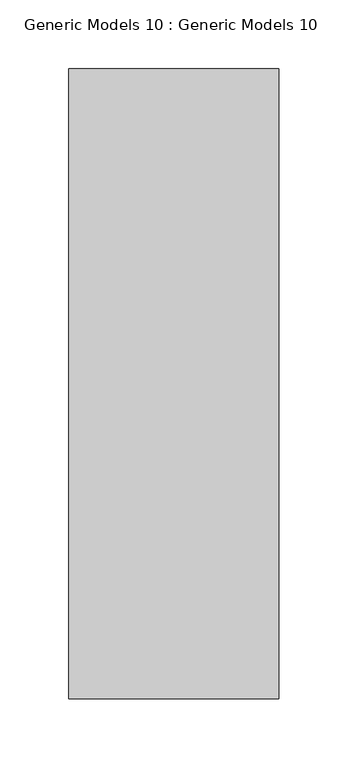
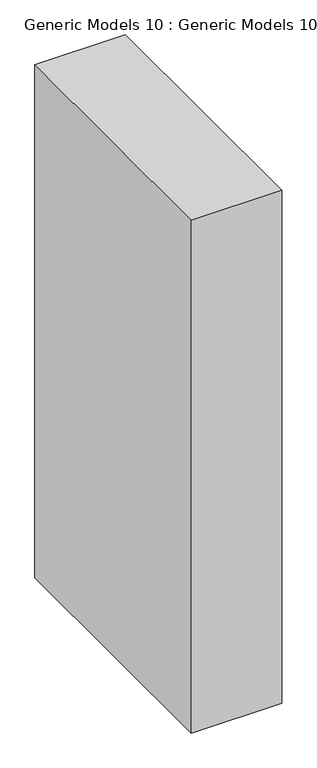
"""IFC4 building model written with IfcOpenShell, lengths in millimetres: proxy geometry, Generic Models 10 : Generic Models 10."""

from ifc_helpers import new_model, si_unit, frame, origin, place, context, project, spatial, polyline, outline, extrude, source, transform, mapped, element, save


def generic_models_10_generic_models_10_3c4deb4f(model_context):
    return source(origin(), model_context, "Body", "SweptSolid", [
        extrude(outline(polyline([(-8551.7906521, -12127.0453012), (-8551.7906521, -11669.8453012), (-8399.3906521, -11669.8453012), (-8399.3906521, -12127.0453012), (-8551.7906521, -12127.0453012)])), frame((0.0, 0.0, 6096.0), z_axis=(0.0, 0.0, 1.0), x_axis=(1.0, 0.0, 0.0)), (0.0, 0.0, 1.0), 914.4),
    ])


if __name__ == "__main__":
    model = new_model("IFC4")
    model_context = context("Model", 3, world=origin())
    ifc_project = project(units=[si_unit("LENGTHUNIT", "METRE", prefix="MILLI")], contexts=[model_context])
    site = spatial("IfcSite", under=ifc_project)
    building = spatial("IfcBuilding", under=site)
    placement = place(None, origin())
    generic_models_10_generic_models_10_shape = generic_models_10_generic_models_10_3c4deb4f(model_context)
    element("IfcBuildingElementProxy", 1, Name="Generic Models 10 : Generic Models 10", ObjectType="Generic Models 10 : Generic Models 10", at=placement, inside=building, context=model_context, shape_type="MappedRepresentation", body=[
        mapped(generic_models_10_generic_models_10_shape, transform((0.0, 0.0, 0.0), x_axis=(1.0, 0.0, 0.0), y_axis=(0.0, 1.0, 0.0), z_axis=(0.0, 0.0, 1.0))),
    ])
    save(model, "model.ifc")

# Revit data of these elements
# Element 1 (IfcBuildingElementProxy, "Generic Models 10 : Generic Models 10")
#   Materials on its faces: "GREY COLOUR FRAME"
# Materials
#   "GREY COLOUR FRAME": class "Generic", colour RGB 120 120 120, transparency 0, Cost = 0
